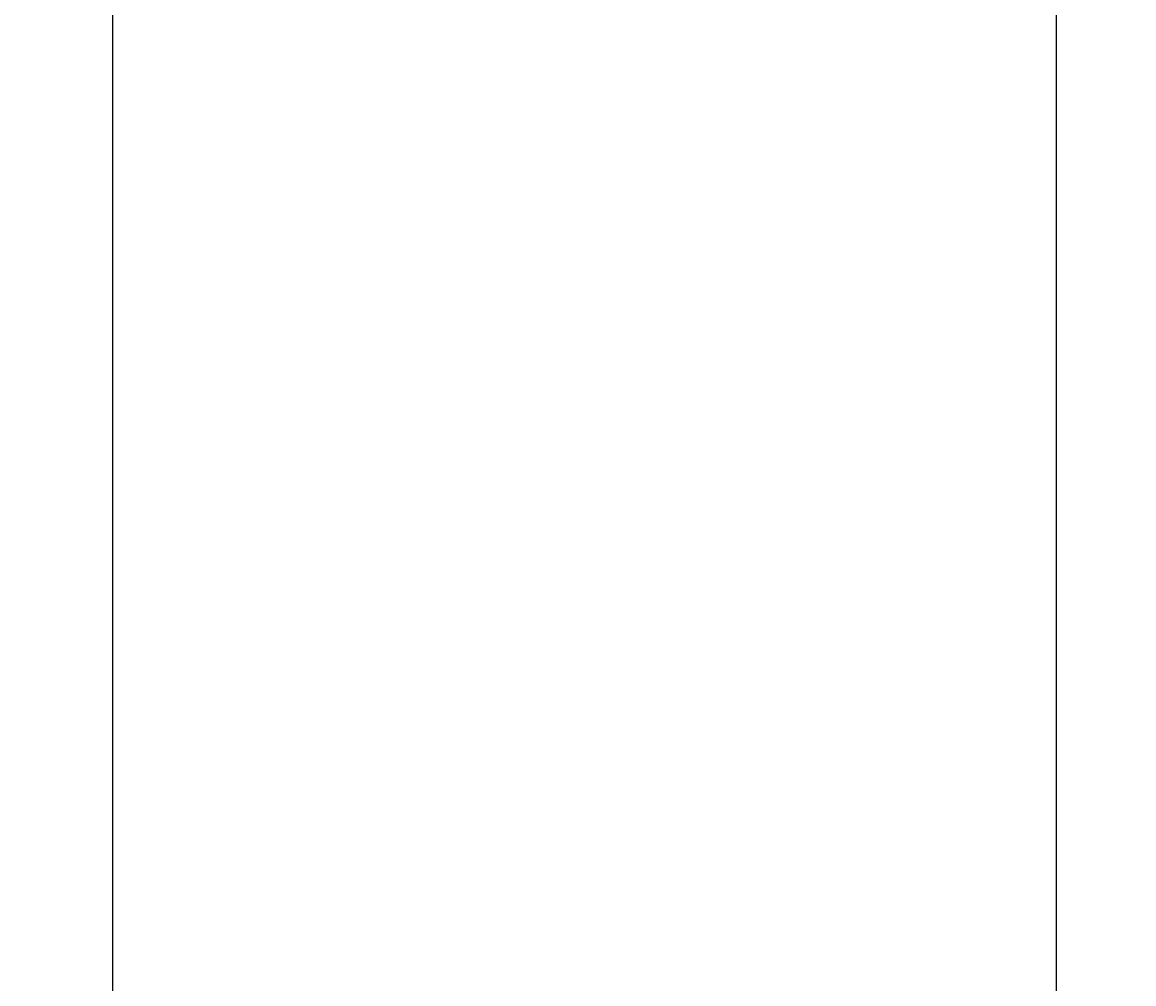
# Model space of a CAD drawing. Units: feet. Extents: x 105 to 1094, y -88 to 588.
# Tile 48 of 59: x 551 to 575, y 492 to 513. Entities that reach past the tile are written whole.
import ezdxf

# ---------------------------------------------------------------- set-up
doc = ezdxf.new("R2010")
doc.units = ezdxf.units.FT
doc.header["$MEASUREMENT"] = 0
doc.layers.add('A-ANNO-DIMS', color=2, linetype='Continuous', lineweight=18)
doc.styles.get("Standard").update_dxf_attribs({"font": 'arial.ttf'})
doc.dimstyles.get("Standard").update_dxf_attribs({"dimtxt": 0.18, "dimasz": 0.18, "dimexe": 0.18, "dimexo": 0.0625, "dimgap": 0.09, "dimtad": 0, "dimtih": 1, "dimtoh": 1, "dimdec": 4, "dimzin": 0, "dimdsep": 46, "dimtxsty": 'Standard', "dimcen": 0.09, "dimadec": 0, "dimazin": 0, "dimtfac": 1, "dimtdec": 4, "dimtofl": 0, "dimtmove": 0, "dimatfit": 3, "dimfxl": 1, "dimtolj": 1, "dimtzin": 0, "dimarcsym": 0})

# ---------------------------------------------------------------- blocks, each defined once
blk = doc.blocks.new('*D21')
at = {"layer": 'A-ANNO-DIMS', "color": 0, "lineweight": -2, "transparency": 16777216}
for p, q in [((849.626, 543.081), (105.458, 543.081)), ((105.638, 542.901), (105.638, 250.263)), ((105.638, -42.739), (105.638, 249.899)), ((849.626, -42.919), (105.458, -42.919))]:
    blk.add_line(p, q, dxfattribs=at)
at = {"layer": 'A-ANNO-DIMS', "color": 0, "transparency": 16777216}
for points in [[(105.608, 542.901), (105.668, 542.901), (105.638, 543.081)], [(105.608, -42.739), (105.668, -42.739), (105.638, -42.919)]]:
    blk.add_solid(points, dxfattribs=at)
at = {"layer": 'Defpoints', "color": 0, "transparency": 16777216}
for p in [(105.638, 543.081), (849.688, 543.081), (849.688, -42.919)]:
    blk.add_point(p, dxfattribs=at)
at = {"layer": 'A-ANNO-DIMS', "color": 0, "transparency": 16777216, "insert": (105.638, 250.081), "char_height": 0.18, "attachment_point": 5}
blk.add_mtext('\\A1;586', dxfattribs=at)
blk = doc.blocks.new('*D25')
at = {"layer": 'A-ANNO-DIMS', "color": 0, "lineweight": -2, "transparency": 16777216}
for p, q in [((438.688, 527.144), (438.688, 588.311)), ((552.688, 471.144), (552.688, 588.311)), ((438.868, 588.131), (495.408, 588.131)), ((552.508, 588.131), (495.968, 588.131))]:
    blk.add_line(p, q, dxfattribs=at)
at = {"layer": 'A-ANNO-DIMS', "color": 0, "transparency": 16777216}
for points in [[(438.868, 588.161), (438.868, 588.101), (438.688, 588.131)], [(552.508, 588.161), (552.508, 588.101), (552.688, 588.131)]]:
    blk.add_solid(points, dxfattribs=at)
at = {"layer": 'Defpoints', "color": 0, "transparency": 16777216}
for p in [(552.688, 588.131), (438.688, 527.081), (552.688, 471.081)]:
    blk.add_point(p, dxfattribs=at)
at = {"layer": 'A-ANNO-DIMS', "color": 0, "transparency": 16777216, "insert": (495.688, 588.131), "char_height": 0.18, "attachment_point": 5}
blk.add_mtext('\\A1;114', dxfattribs=at)
blk = doc.blocks.new('*D26')
at = {"layer": 'A-ANNO-DIMS', "color": 0, "lineweight": -2, "transparency": 16777216}
for p, q in [((552.688, 471.144), (552.688, 588.311)), ((646.688, 471.144), (646.688, 588.311)), ((552.868, 588.131), (599.47, 588.131)), ((646.508, 588.131), (599.907, 588.131))]:
    blk.add_line(p, q, dxfattribs=at)
at = {"layer": 'A-ANNO-DIMS', "color": 0, "transparency": 16777216}
for points in [[(552.868, 588.161), (552.868, 588.101), (552.688, 588.131)], [(646.508, 588.161), (646.508, 588.101), (646.688, 588.131)]]:
    blk.add_solid(points, dxfattribs=at)
at = {"layer": 'Defpoints', "color": 0, "transparency": 16777216}
for p in [(646.688, 588.131), (552.688, 471.081), (646.688, 471.081)]:
    blk.add_point(p, dxfattribs=at)
at = {"layer": 'A-ANNO-DIMS', "color": 0, "transparency": 16777216, "insert": (599.688, 588.131), "char_height": 0.18, "attachment_point": 5}
blk.add_mtext('\\A1;94', dxfattribs=at)
blk = doc.blocks.new('*D31')
at = {"layer": 'A-ANNO-DIMS', "color": 0, "lineweight": -2, "transparency": 16777216}
for p, q in [((438.751, 527.081), (1093.918, 527.081)), ((1093.738, 526.901), (1093.738, 499.263)), ((1093.738, 471.261), (1093.738, 498.899)), ((438.751, 471.081), (1093.918, 471.081))]:
    blk.add_line(p, q, dxfattribs=at)
at = {"layer": 'A-ANNO-DIMS', "color": 0, "transparency": 16777216}
for points in [[(1093.708, 526.901), (1093.768, 526.901), (1093.738, 527.081)], [(1093.708, 471.261), (1093.768, 471.261), (1093.738, 471.081)]]:
    blk.add_solid(points, dxfattribs=at)
at = {"layer": 'Defpoints', "color": 0, "transparency": 16777216}
for p in [(438.688, 527.081), (1093.738, 527.081), (438.688, 471.081)]:
    blk.add_point(p, dxfattribs=at)
at = {"layer": 'A-ANNO-DIMS', "color": 0, "transparency": 16777216, "insert": (1093.738, 499.081), "char_height": 0.18, "attachment_point": 5}
blk.add_mtext('\\A1;56', dxfattribs=at)
blk = doc.blocks.new('*D47')
at = {"layer": 'A-ANNO-DIMS', "color": 0, "lineweight": -2, "transparency": 16777216}
for p, q in [((552.688, 441.144), (552.688, 588.311)), ((573.483, 441.144), (573.483, 588.311)), ((552.868, 588.131), (562.621, 588.131)), ((573.303, 588.131), (563.55, 588.131))]:
    blk.add_line(p, q, dxfattribs=at)
at = {"layer": 'A-ANNO-DIMS', "color": 0, "transparency": 16777216}
for points in [[(552.868, 588.161), (552.868, 588.101), (552.688, 588.131)], [(573.303, 588.161), (573.303, 588.101), (573.483, 588.131)]]:
    blk.add_solid(points, dxfattribs=at)
at = {"layer": 'Defpoints', "color": 0, "transparency": 16777216}
for p in [(573.483, 588.131), (552.688, 441.081), (573.483, 441.081)]:
    blk.add_point(p, dxfattribs=at)
at = {"layer": 'A-ANNO-DIMS', "color": 0, "transparency": 16777216, "insert": (563.085, 588.131), "char_height": 0.18, "attachment_point": 5}
blk.add_mtext('\\A1;20.794', dxfattribs=at)
blk = doc.blocks.new('*D48')
at = {"layer": 'A-ANNO-DIMS', "color": 0, "lineweight": -2, "transparency": 16777216}
for p, q in [((573.483, 441.144), (573.483, 588.311)), ((633.483, 441.144), (633.483, 588.311)), ((573.663, 588.131), (603.263, 588.131)), ((633.303, 588.131), (603.702, 588.131))]:
    blk.add_line(p, q, dxfattribs=at)
at = {"layer": 'A-ANNO-DIMS', "color": 0, "transparency": 16777216}
for points in [[(573.663, 588.161), (573.663, 588.101), (573.483, 588.131)], [(633.303, 588.161), (633.303, 588.101), (633.483, 588.131)]]:
    blk.add_solid(points, dxfattribs=at)
at = {"layer": 'Defpoints', "color": 0, "transparency": 16777216}
for p in [(633.483, 588.131), (573.483, 441.081), (633.483, 441.081)]:
    blk.add_point(p, dxfattribs=at)
at = {"layer": 'A-ANNO-DIMS', "color": 0, "transparency": 16777216, "insert": (603.483, 588.131), "char_height": 0.18, "attachment_point": 5}
blk.add_mtext('\\A1;60', dxfattribs=at)

msp = doc.modelspace()

# ---------------------------------------------------------------- dimensions: what is measured, and where the dimension line sits
at = {"layer": 'A-ANNO-DIMS'}
for base, p1, p2, override, picture, middle in [((552.6883, 588.1312), (438.6883, 527.0812), (552.6883, 471.0812), {"dimdec": 0, "dimlfac": 1, "dimrnd": 0, "dimzin": 0, "dimdsep": 46, "dimlunit": 2}, '*D25', (495.6883, 588.1312)), ((646.6883, 588.1312), (552.6883, 471.0812), (646.6883, 471.0812), {"dimdec": 0, "dimlfac": 1, "dimrnd": 0, "dimzin": 0, "dimdsep": 46, "dimlunit": 2}, '*D26', (599.6883, 588.1312)), ((573.4826, 588.1312), (552.6883, 441.0812), (573.4826, 441.0812), {"dimdec": 3, "dimlfac": 1, "dimrnd": 0, "dimzin": 0, "dimdsep": 46, "dimlunit": 2}, '*D47', (563.0854, 588.1312)), ((633.4826, 588.1312), (573.4826, 441.0812), (633.4826, 441.0812), {"dimdec": 0, "dimlfac": 1, "dimrnd": 0, "dimzin": 0, "dimdsep": 46, "dimlunit": 2}, '*D48', (603.4826, 588.1312))]:
    dim = msp.add_linear_dim(base=base, p1=p1, p2=p2, dimstyle='Standard', override=override, dxfattribs=at)
    dim.commit()
    dim.dimension.update_dxf_attribs({"geometry": picture, "text_midpoint": middle})
for base, p1, p2, picture, middle in [((105.6383, 543.0812), (849.6883, -42.9188), (849.6883, 543.0812), '*D21', (105.6383, 250.0812)), ((1093.7383, 527.0812), (438.6883, 471.0812), (438.6883, 527.0812), '*D31', (1093.7383, 499.0812))]:
    dim = msp.add_linear_dim(base=base, p1=p1, p2=p2, angle=90, dimstyle='Standard', override={"dimdec": 0, "dimlfac": 1, "dimrnd": 0, "dimzin": 0, "dimdsep": 46, "dimlunit": 2}, dxfattribs=at)
    dim.commit()
    dim.dimension.update_dxf_attribs({"geometry": picture, "text_midpoint": middle})

doc.saveas('drawing.dxf')
